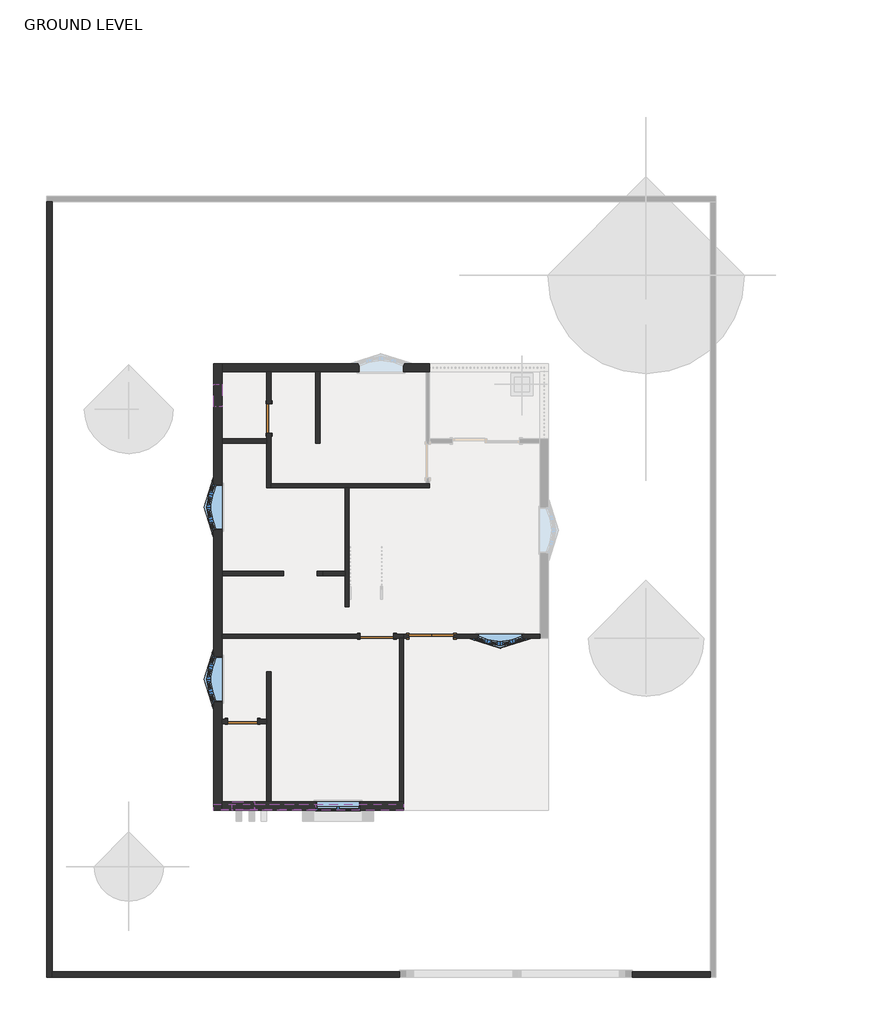
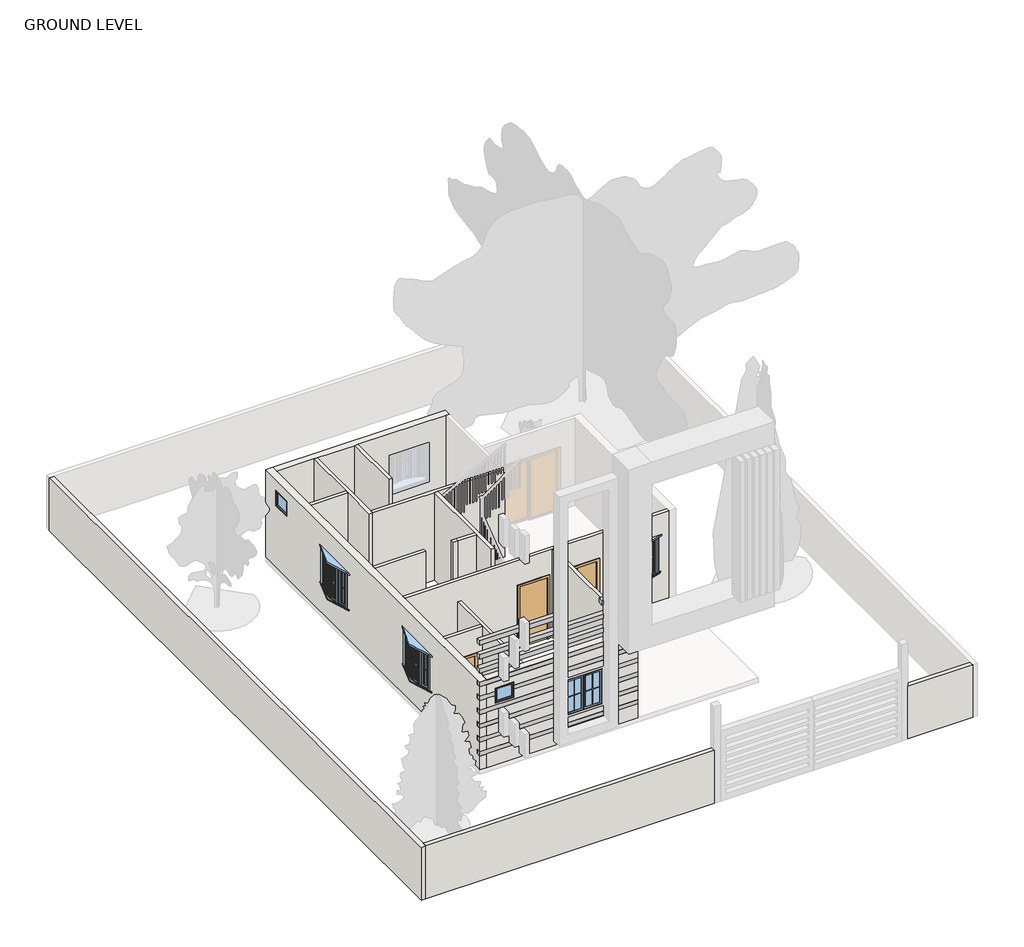
# One storey, part 1 of 3: 19 walls, 9 proxies, 6 windows, 4 doors.
"""IFC4 building model written with IfcOpenShell, lengths in millimetres."""

from ifc_helpers import new_model, si_unit, frame, origin, origin_with_axes, place, context, project, spatial, polyline, outline, extrude, faceted_brep, transform, mapped, element, save
from components import door_double_flush_panel_4_x7_eb8a45e1, door_d141acb4, door_38851409, single_flush_3_x7_305aa2a5, window_9e637e28, window_bow_casement_10_degree_angle_4_x4_fc1e5cf1, window_bow_casement_10_degree_angle_4_x4_a8433a54, window_casement_double_4_x4_af3140d2

model = new_model("IFC4")

# Units and contexts
model_context = context("Model", 3, world=origin())
ifc_project = project(units=[si_unit("LENGTHUNIT", "METRE", prefix="MILLI")], contexts=[model_context])

# Site, building, storey
site = spatial("IfcSite", under=ifc_project)
building = spatial("IfcBuilding", under=site)
storey = spatial("IfcBuildingStorey", under=building, Name="GROUND LEVEL", Elevation=0.0)

# Proxies
placement = place(None, origin())
element("IfcBuildingElementProxy", 1, Name="Reveal", ObjectType="Reveal", at=placement, inside=storey, context=model_context, shape_type="SweptSolid", body=[
    extrude(outline(polyline([(-1823.7720223, -5557.8064015), (-1823.7720223, -5405.4064015), (-645.6415084, -5405.4064015), (-645.6415084, -5557.8064015), (-1823.7720223, -5557.8064015)])), frame((0.0, 0.0, 4331.3684211), z_axis=(0.0, 0.0, 1.0), x_axis=(1.0, 0.0, 0.0)), (0.0, 0.0, 1.0), 152.4),
    extrude(outline(polyline([(-5827.2415084, -5557.8064015), (-5827.2415084, -5405.4064015), (-3042.9720223, -5405.4064015), (-3042.9720223, -5557.8064015), (-5827.2415084, -5557.8064015)])), frame((0.0, 0.0, 4331.3684211), z_axis=(0.0, 0.0, 1.0), x_axis=(1.0, 0.0, 0.0)), (0.0, 0.0, 1.0), 152.4),
])
element("IfcBuildingElementProxy", 2, Name="Reveal", ObjectType="Reveal", at=placement, inside=storey, context=model_context, shape_type="SweptSolid", body=[
    extrude(outline(polyline([(-5827.2415084, -5557.8064015), (-5827.2415084, -5405.4064015), (-645.6415084, -5405.4064015), (-645.6415084, -5557.8064015), (-5827.2415084, -5557.8064015)])), frame((0.0, 0.0, 3850.1052632), z_axis=(0.0, 0.0, 1.0), x_axis=(1.0, 0.0, 0.0)), (0.0, 0.0, 1.0), 152.4),
])
element("IfcBuildingElementProxy", 3, Name="Reveal", ObjectType="Reveal", at=placement, inside=storey, context=model_context, shape_type="SweptSolid", body=[
    extrude(outline(polyline([(-5827.2415084, -5557.8064015), (-5827.2415084, -5405.4064015), (-645.6415084, -5405.4064015), (-645.6415084, -5557.8064015), (-5827.2415084, -5557.8064015)])), frame((0.0, 0.0, 3368.8421053), z_axis=(0.0, 0.0, 1.0), x_axis=(1.0, 0.0, 0.0)), (0.0, 0.0, 1.0), 152.4),
])
element("IfcBuildingElementProxy", 4, Name="Reveal", ObjectType="Reveal", at=placement, inside=storey, context=model_context, shape_type="SweptSolid", body=[
    extrude(outline(polyline([(-5827.2415084, -5557.8064015), (-5827.2415084, -5405.4064015), (-645.6415084, -5405.4064015), (-645.6415084, -5557.8064015), (-5827.2415084, -5557.8064015)])), frame((0.0, 0.0, 2887.5789474), z_axis=(0.0, 0.0, 1.0), x_axis=(1.0, 0.0, 0.0)), (0.0, 0.0, 1.0), 152.4),
])
element("IfcBuildingElementProxy", 5, Name="Reveal", ObjectType="Reveal", at=placement, inside=storey, context=model_context, shape_type="SweptSolid", body=[
    extrude(outline(polyline([(-4712.8165084, -5557.8064015), (-4712.8165084, -5405.4064015), (-645.6415084, -5405.4064015), (-645.6415084, -5557.8064015), (-4712.8165084, -5557.8064015)])), frame((0.0, 0.0, 2406.3157895), z_axis=(0.0, 0.0, 1.0), x_axis=(1.0, 0.0, 0.0)), (0.0, 0.0, 1.0), 152.4),
    extrude(outline(polyline([(-5827.2415084, -5557.8064015), (-5827.2415084, -5405.4064015), (-5322.4165084, -5405.4064015), (-5322.4165084, -5557.8064015), (-5827.2415084, -5557.8064015)])), frame((0.0, 0.0, 2406.3157895), z_axis=(0.0, 0.0, 1.0), x_axis=(1.0, 0.0, 0.0)), (0.0, 0.0, 1.0), 152.4),
])
element("IfcBuildingElementProxy", 6, Name="Reveal", ObjectType="Reveal", at=placement, inside=storey, context=model_context, shape_type="SweptSolid", body=[
    extrude(outline(polyline([(-1823.7720223, -5557.8064015), (-1823.7720223, -5405.4064015), (-645.6415084, -5405.4064015), (-645.6415084, -5557.8064015), (-1823.7720223, -5557.8064015)])), frame((0.0, 0.0, 1925.0526316), z_axis=(0.0, 0.0, 1.0), x_axis=(1.0, 0.0, 0.0)), (0.0, 0.0, 1.0), 152.4),
    extrude(outline(polyline([(-5827.2415084, -5557.8064015), (-5827.2415084, -5405.4064015), (-3042.9720223, -5405.4064015), (-3042.9720223, -5557.8064015), (-5827.2415084, -5557.8064015)])), frame((0.0, 0.0, 1925.0526316), z_axis=(0.0, 0.0, 1.0), x_axis=(1.0, 0.0, 0.0)), (0.0, 0.0, 1.0), 152.4),
])
element("IfcBuildingElementProxy", 7, Name="Reveal", ObjectType="Reveal", at=placement, inside=storey, context=model_context, shape_type="SweptSolid", body=[
    extrude(outline(polyline([(-1823.7720223, -5557.8064015), (-1823.7720223, -5405.4064015), (-645.6415084, -5405.4064015), (-645.6415084, -5557.8064015), (-1823.7720223, -5557.8064015)])), frame((0.0, 0.0, 1443.7894737), z_axis=(0.0, 0.0, 1.0), x_axis=(1.0, 0.0, 0.0)), (0.0, 0.0, 1.0), 152.4),
    extrude(outline(polyline([(-5827.2415084, -5557.8064015), (-5827.2415084, -5405.4064015), (-3042.9720223, -5405.4064015), (-3042.9720223, -5557.8064015), (-5827.2415084, -5557.8064015)])), frame((0.0, 0.0, 1443.7894737), z_axis=(0.0, 0.0, 1.0), x_axis=(1.0, 0.0, 0.0)), (0.0, 0.0, 1.0), 152.4),
])
element("IfcBuildingElementProxy", 8, Name="Reveal", ObjectType="Reveal", at=placement, inside=storey, context=model_context, shape_type="SweptSolid", body=[
    extrude(outline(polyline([(-5827.2415084, -5557.8064015), (-5827.2415084, -5405.4064015), (-3042.9720223, -5405.4064015), (-3042.9720223, -5557.8064015), (-5827.2415084, -5557.8064015)])), frame((0.0, 0.0, 962.5263158), z_axis=(0.0, 0.0, 1.0), x_axis=(1.0, 0.0, 0.0)), (0.0, 0.0, 1.0), 152.4),
    extrude(outline(polyline([(-1823.7720223, -5557.8064015), (-1823.7720223, -5405.4064015), (-645.6415084, -5405.4064015), (-645.6415084, -5557.8064015), (-1823.7720223, -5557.8064015)])), frame((0.0, 0.0, 962.5263158), z_axis=(0.0, 0.0, 1.0), x_axis=(1.0, 0.0, 0.0)), (0.0, 0.0, 1.0), 152.4),
])
element("IfcBuildingElementProxy", 9, Name="Reveal", ObjectType="Reveal", at=placement, inside=storey, context=model_context, shape_type="SweptSolid", body=[
    extrude(outline(polyline([(-5827.2415084, -5557.8064015), (-5827.2415084, -5405.4064015), (-645.6415084, -5405.4064015), (-645.6415084, -5557.8064015), (-5827.2415084, -5557.8064015)])), frame((0.0, 0.0, 481.2631579), z_axis=(0.0, 0.0, 1.0), x_axis=(1.0, 0.0, 0.0)), (0.0, 0.0, 1.0), 152.4),
])

# Doors
door_double_flush_panel_4_x7_shape = door_double_flush_panel_4_x7_eb8a45e1(model_context)
element("IfcDoor", 10, ObjectType="Door-Double-Flush_Panel : 4'X7'", at=placement, inside=storey, context=model_context, shape_type="MappedRepresentation", body=[
    mapped(door_double_flush_panel_4_x7_shape, transform((116.3584916, -814.3564015, 0.0), x_axis=(1.0, 0.0, 0.0), y_axis=(0.0, 1.0, 0.0), z_axis=(0.0, 0.0, 1.0))),
])
door_shape = door_d141acb4(model_context)
element("IfcDoor", 11, ObjectType="Single-Flush : 2'8\"X7'", at=placement, inside=storey, context=model_context, shape_type="MappedRepresentation", body=[
    mapped(door_shape, transform((-5039.8415084, -3138.4564015, 0.0), x_axis=(-1.0, 0.0, 0.0), y_axis=(0.0, -1.0, 0.0), z_axis=(0.0, 0.0, 1.0))),
])
door_2_shape = door_38851409(model_context)
element("IfcDoor", 12, ObjectType="Single-Flush : 2'8\"X7'", at=placement, inside=storey, context=model_context, shape_type="MappedRepresentation", body=[
    mapped(door_2_shape, transform((-4322.2915084, 5135.5935985, 0.0), x_axis=(0.0, -1.0, 0.0), y_axis=(1.0, 0.0, 0.0), z_axis=(0.0, 0.0, 1.0))),
])
single_flush_3_x7_shape = single_flush_3_x7_305aa2a5(model_context)
element("IfcDoor", 13, ObjectType="Single-Flush : 3'X7'", at=placement, inside=storey, context=model_context, shape_type="MappedRepresentation", body=[
    mapped(single_flush_3_x7_shape, transform((-1369.5415084, -814.3564015, 0.0), x_axis=(1.0, 0.0, 0.0), y_axis=(0.0, 1.0, 0.0), z_axis=(0.0, 0.0, 1.0))),
])

# Walls
element("IfcWall", 14, ObjectType="4.5\"", at=placement, inside=storey, context=model_context, shape_type="Brep", body=[
    faceted_brep([(-912.3415084, -871.5064015, 2133.6), (-912.3415084, -871.5064015, 0.0), (-759.9415084, -871.5064015, 0.0), (-645.6415084, -871.5064015, 0.0), (-645.6415084, -871.5064015, 3048.0), (-759.9415084, -871.5064015, 3048.0), (-5598.6415084, -871.5064015, 3048.0), (-5598.6415084, -871.5064015, 0.0), (-1826.7415084, -871.5064015, 0.0), (-1826.7415084, -871.5064015, 2133.6), (-645.6415084, -757.2064015, 0.0), (-912.3415084, -757.2064015, 0.0), (-912.3415084, -757.2064015, 2133.6), (-1826.7415084, -757.2064015, 2133.6), (-1826.7415084, -757.2064015, 0.0), (-5598.6415084, -757.2064015, 0.0), (-5598.6415084, -757.2064015, 3048.0), (-645.6415084, -757.2064015, 3048.0)], [[[0, 1, 2, 3, 4, 5, 6, 7, 8, 9]], [[10, 11, 12, 13, 14, 15, 16, 17]], [[8, 7, 15, 14]], [[3, 2, 1, 11, 10]], [[6, 5, 4, 17, 16]], [[7, 6, 16, 15]], [[4, 3, 10, 17]], [[12, 11, 1, 0]], [[13, 12, 0, 9]], [[14, 13, 9, 8]]]),
])
element("IfcWall", 15, ObjectType="4.5\"", at=placement, inside=storey, context=model_context, shape_type="SweptSolid", body=[
    extrude(outline(polyline([(-759.9415084, -5329.2064015), (-759.9415084, -871.5064015), (-645.6415084, -871.5064015), (-645.6415084, -5329.2064015), (-759.9415084, -5329.2064015)])), origin_with_axes(), (0.0, 0.0, 1.0), 3048.0),
])
element("IfcWall", 16, ObjectType="4.5\"", at=placement, inside=storey, context=model_context, shape_type="Brep", body=[
    faceted_brep([(-645.6415084, -757.2064015, 3048.0), (3088.1584916, -757.2064015, 3048.0), (3088.1584916, -757.2064015, 0.0), (725.9584916, -757.2064015, 0.0), (725.9584916, -757.2064015, 2133.6), (-493.2415084, -757.2064015, 2133.6), (-493.2415084, -757.2064015, 0.0), (-645.6415084, -757.2064015, 0.0), (2603.2834745, -757.2064015, 2263.7323709), (1384.0834745, -757.2064015, 2263.7323709), (1384.0834745, -757.2064015, 993.7323709), (2603.2834745, -757.2064015, 993.7323709), (3088.1584916, -871.5064015, 3048.0), (-645.6415084, -871.5064015, 3048.0), (-645.6415084, -871.5064015, 0.0), (-493.2415084, -871.5064015, 0.0), (-493.2415084, -871.5064015, 2133.6), (725.9584916, -871.5064015, 2133.6), (725.9584916, -871.5064015, 0.0), (3088.1584916, -871.5064015, 0.0), (1360.1933675, -871.5064015, 2263.7323709), (2627.1735815, -871.5064015, 2263.7323709), (2627.1735815, -871.5064015, 993.7323709), (1360.1933675, -871.5064015, 993.7323709), (2603.2834745, -805.868872, 2263.7323709), (1384.0834745, -805.868872, 2263.7323709), (2603.2834745, -805.868872, 993.7323709), (1384.0834745, -805.868872, 993.7323709)], [[[0, 1, 2, 3, 4, 5, 6, 7], [8, 9, 10, 11]], [[12, 13, 14, 15, 16, 17, 18, 19], [20, 21, 22, 23]], [[2, 19, 18, 3]], [[14, 7, 6, 15]], [[1, 0, 13, 12]], [[2, 1, 12, 19]], [[0, 7, 14, 13]], [[17, 4, 3, 18]], [[4, 17, 16, 5]], [[5, 16, 15, 6]], [[24, 21, 20, 25, 9, 8]], [[26, 11, 10, 27, 23, 22]], [[24, 8, 11, 26]], [[9, 25, 27, 10]], [[25, 20, 23, 27]], [[21, 24, 26, 22]]]),
])
element("IfcWall", 17, ObjectType="4.5\"", at=placement, inside=storey, context=model_context, shape_type="SweptSolid", body=[
    extrude(outline(polyline([(-3045.9415084, 4462.4935985), (-3045.9415084, 6405.5935985), (-2931.6415084, 6405.5935985), (-2931.6415084, 4462.4935985), (-3045.9415084, 4462.4935985)])), origin_with_axes(), (0.0, 0.0, 1.0), 3048.0),
])
element("IfcWall", 18, ObjectType="4.5\"", at=placement, inside=storey, context=model_context, shape_type="Brep", body=[
    faceted_brep([(-4379.4415084, 4729.1935985, 2133.6), (-4379.4415084, 4729.1935985, 0.0), (-4379.4415084, 4576.7935985, 0.0), (-4379.4415084, 4462.4935985, 0.0), (-4379.4415084, 3243.2935985, 0.0), (-4379.4415084, 3243.2935985, 3048.0), (-4379.4415084, 4462.4935985, 3048.0), (-4379.4415084, 4576.7935985, 3048.0), (-4379.4415084, 6405.5935985, 3048.0), (-4379.4415084, 6405.5935985, 0.0), (-4379.4415084, 5541.9935985, 0.0), (-4379.4415084, 5541.9935985, 2133.6), (-4265.1415084, 3243.2935985, 0.0), (-4265.1415084, 3357.5935985, 0.0), (-4265.1415084, 4729.1935985, 0.0), (-4265.1415084, 4729.1935985, 2133.6), (-4265.1415084, 5541.9935985, 2133.6), (-4265.1415084, 5541.9935985, 0.0), (-4265.1415084, 6405.5935985, 0.0), (-4265.1415084, 6405.5935985, 3048.0), (-4265.1415084, 3357.5935985, 3048.0), (-4265.1415084, 3243.2935985, 3048.0)], [[[0, 1, 2, 3, 4, 5, 6, 7, 8, 9, 10, 11]], [[12, 13, 14, 15, 16, 17, 18, 19, 20, 21]], [[10, 9, 18, 17]], [[4, 3, 2, 1, 14, 13, 12]], [[8, 7, 6, 5, 21, 20, 19]], [[9, 8, 19, 18]], [[5, 4, 12, 21]], [[15, 14, 1, 0]], [[16, 15, 0, 11]], [[17, 16, 11, 10]]]),
])
element("IfcWall", 19, ObjectType="4.5\"", at=placement, inside=storey, context=model_context, shape_type="SweptSolid", body=[
    extrude(outline(polyline([(-5598.6415084, 4576.7935985), (-4379.4415084, 4576.7935985), (-4379.4415084, 4462.4935985), (-5598.6415084, 4462.4935985), (-5598.6415084, 4576.7935985)])), origin_with_axes(), (0.0, 0.0, 1.0), 3048.0),
])
element("IfcWall", 20, ObjectType="4.5\"", at=placement, inside=storey, context=model_context, shape_type="Brep", body=[
    faceted_brep([(-4265.1415084, 3243.2935985, 0.0), (-2245.8415084, 3243.2935985, 0.0), (-2131.5415084, 3243.2935985, 0.0), (65.5584916, 3243.2935985, 0.0), (65.5584916, 3243.2935985, 3048.0), (-2131.5415084, 3243.2935985, 3048.0), (-2245.8415084, 3243.2935985, 3048.0), (-4265.1415084, 3243.2935985, 3048.0), (-4265.1415084, 3357.5935985, 0.0), (-4265.1415084, 3357.5935985, 3048.0), (-36.0415084, 3357.5935985, 3048.0), (65.5584916, 3357.5935985, 3048.0), (65.5584916, 3357.5935985, 0.0), (-36.0415084, 3357.5935985, 0.0)], [[[0, 1, 2, 3, 4, 5, 6, 7]], [[8, 9, 10, 11, 12, 13]], [[3, 2, 1, 0, 8, 13, 12]], [[7, 6, 5, 4, 11, 10, 9]], [[0, 7, 9, 8]], [[4, 3, 12, 11]]]),
])
element("IfcWall", 21, ObjectType="4.5\"", at=placement, inside=storey, context=model_context, shape_type="SweptSolid", body=[
    extrude(outline(polyline([(-3922.2415084, 842.9935985), (-5598.6415084, 842.9935985), (-5598.6415084, 957.2935985), (-3922.2415084, 957.2935985), (-3922.2415084, 842.9935985)])), origin_with_axes(), (0.0, 0.0, 1.0), 3048.0),
])
element("IfcWall", 22, ObjectType="4.5\"", at=placement, inside=storey, context=model_context, shape_type="SweptSolid", body=[
    extrude(outline(polyline([(-3007.8415084, 957.2935985), (-2855.4415084, 957.2935985), (-2855.4415084, 842.9935985), (-3007.8415084, 842.9935985), (-3007.8415084, 957.2935985)])), origin_with_axes(), (0.0, 0.0, 1.0), 3048.0),
])
element("IfcWall", 23, ObjectType="4.5\"", at=placement, inside=storey, context=model_context, shape_type="Brep", body=[
    faceted_brep([(-2245.8415084, 3243.2935985, 0.0), (-2245.8415084, 957.2935985, 0.0), (-2245.8415084, 842.9935985, 0.0), (-2245.8415084, -9.4533727, 0.0), (-2245.8415084, -9.4533727, 3048.0), (-2245.8415084, 842.9935985, 3048.0), (-2245.8415084, 957.2935985, 3048.0), (-2245.8415084, 3243.2935985, 3048.0), (-2131.5415084, 3243.2935985, 0.0), (-2131.5415084, 3243.2935985, 3048.0), (-2131.5415084, -9.4533727, 3048.0), (-2131.5415084, -9.4533727, 0.0)], [[[0, 1, 2, 3, 4, 5, 6, 7]], [[8, 9, 10, 11]], [[3, 2, 1, 0, 8, 11]], [[4, 3, 11, 10]], [[7, 6, 5, 4, 10, 9]], [[0, 7, 9, 8]]]),
])
element("IfcWall", 24, ObjectType="4.5\"", at=placement, inside=storey, context=model_context, shape_type="SweptSolid", body=[
    extrude(outline(polyline([(-2245.8415084, 842.9935985), (-2855.4415084, 842.9935985), (-2855.4415084, 957.2935985), (-2245.8415084, 957.2935985), (-2245.8415084, 842.9935985)])), origin_with_axes(), (0.0, 0.0, 1.0), 3048.0),
])
element("IfcWall", 25, ObjectType="4.5\"", at=placement, inside=storey, context=model_context, shape_type="Brep", body=[
    faceted_brep([(-4265.1415084, -5329.2064015, 0.0), (-4265.1415084, -1785.9064015, 0.0), (-4265.1415084, -1785.9064015, 3048.0), (-4265.1415084, -5329.2064015, 3048.0), (-4379.4415084, -5329.2064015, 0.0), (-4379.4415084, -5329.2064015, 3048.0), (-4379.4415084, -3195.6064015, 3048.0), (-4379.4415084, -3081.3064015, 3048.0), (-4379.4415084, -1785.9064015, 3048.0), (-4379.4415084, -1785.9064015, 0.0), (-4379.4415084, -3081.3064015, 0.0), (-4379.4415084, -3195.6064015, 0.0)], [[[0, 1, 2, 3]], [[4, 5, 6, 7, 8, 9, 10, 11]], [[1, 0, 4, 11, 10, 9]], [[2, 1, 9, 8]], [[3, 2, 8, 7, 6, 5]], [[0, 3, 5, 4]]]),
])
element("IfcWall", 26, ObjectType="4.5\"", at=placement, inside=storey, context=model_context, shape_type="SweptSolid", body=[
    extrude(outline(polyline([(0.0, -5598.6415084), (0.0, -5446.2415084), (2133.6, -5446.2415084), (2133.6, -4633.4415084), (0.0, -4633.4415084), (0.0, -4379.4415084), (3048.0, -4379.4415084), (3048.0, -5598.6415084), (0.0, -5598.6415084)])), frame((0.0, -3195.6064015, 0.0), z_axis=(0.0, 1.0, 0.0), x_axis=(0.0, 0.0, 1.0)), (0.0, 0.0, 1.0), 114.3),
])
element("IfcWall", 27, ObjectType="6\"", at=placement, inside=storey, context=model_context, shape_type="Brep", body=[
    faceted_brep([(-10399.2415084, 11053.7935985, -152.4), (-10399.2415084, -10129.8064015, -152.4), (-10399.2415084, -10129.8064015, 1676.4), (-10399.2415084, 11053.7935985, 1676.4), (-10246.8415084, 11053.7935985, -152.4), (-10246.8415084, 11053.7935985, 1676.4), (-10246.8415084, -9977.4064015, 1676.4), (-10246.8415084, -10129.8064015, 1676.4), (-10246.8415084, -10129.8064015, -152.4), (-10246.8415084, -9977.4064015, -152.4)], [[[0, 1, 2, 3]], [[4, 5, 6, 7, 8, 9]], [[1, 0, 4, 9, 8]], [[3, 2, 7, 6, 5]], [[0, 3, 5, 4]], [[2, 1, 8, 7]]]),
])
element("IfcWall", 28, ObjectType="6\"", at=placement, inside=storey, context=model_context, shape_type="SweptSolid", body=[
    extrude(outline(polyline([(-759.9415084, -10129.8064015), (-10246.8415084, -10129.8064015), (-10246.8415084, -9977.4064015), (-759.9415084, -9977.4064015), (-759.9415084, -10129.8064015)])), frame((0.0, 0.0, -152.4), z_axis=(0.0, 0.0, 1.0), x_axis=(1.0, 0.0, 0.0)), (0.0, 0.0, 1.0), 1828.8),
])
element("IfcWall", 29, ObjectType="6\"", at=placement, inside=storey, context=model_context, shape_type="SweptSolid", body=[
    extrude(outline(polyline([(5602.7584916, -9977.4064015), (7736.3584916, -9977.4064015), (7736.3584916, -10129.8064015), (5602.7584916, -10129.8064015), (5602.7584916, -9977.4064015)])), frame((0.0, 0.0, -152.4), z_axis=(0.0, 0.0, 1.0), x_axis=(1.0, 0.0, 0.0)), (0.0, 0.0, 1.0), 1828.8),
])
element("IfcWall", 30, ObjectType="9\"", at=placement, inside=storey, context=model_context, shape_type="Brep", body=[
    faceted_brep([(-5827.2415084, 6634.1935985, 0.0), (-5827.2415084, -5557.8064015, 0.0), (-5827.2415084, -5557.8064015, 481.2631579), (-5827.2415084, -5405.4064015, 481.2631579), (-5827.2415084, -5405.4064015, 633.6631579), (-5827.2415084, -5557.8064015, 633.6631579), (-5827.2415084, -5557.8064015, 962.5263158), (-5827.2415084, -5405.4064015, 962.5263158), (-5827.2415084, -5405.4064015, 1114.9263158), (-5827.2415084, -5557.8064015, 1114.9263158), (-5827.2415084, -5557.8064015, 1443.7894737), (-5827.2415084, -5405.4064015, 1443.7894737), (-5827.2415084, -5405.4064015, 1596.1894737), (-5827.2415084, -5557.8064015, 1596.1894737), (-5827.2415084, -5557.8064015, 1925.0526316), (-5827.2415084, -5405.4064015, 1925.0526316), (-5827.2415084, -5405.4064015, 2077.4526316), (-5827.2415084, -5557.8064015, 2077.4526316), (-5827.2415084, -5557.8064015, 2406.3157895), (-5827.2415084, -5405.4064015, 2406.3157895), (-5827.2415084, -5405.4064015, 2558.7157895), (-5827.2415084, -5557.8064015, 2558.7157895), (-5827.2415084, -5557.8064015, 2887.5789474), (-5827.2415084, -5405.4064015, 2887.5789474), (-5827.2415084, -5405.4064015, 3039.9789474), (-5827.2415084, -5557.8064015, 3039.9789474), (-5827.2415084, -5557.8064015, 3048.0), (-5827.2415084, 6634.1935985, 3048.0), (-5827.2415084, 6062.6935985, 2133.6), (-5827.2415084, 6062.6935985, 2667.0), (-5827.2415084, 5453.0935985, 2667.0), (-5827.2415084, 5453.0935985, 2133.6), (-5827.2415084, -1354.6176736, 2263.7323709), (-5827.2415084, -2621.5978876, 2263.7323709), (-5827.2415084, -2621.5978876, 993.7323709), (-5827.2415084, -1354.6176736, 993.7323709), (-5827.2415084, 3342.0645075, 2263.7323709), (-5827.2415084, 2075.0842935, 2263.7323709), (-5827.2415084, 2075.0842935, 993.7323709), (-5827.2415084, 3342.0645075, 993.7323709), (-5598.6415084, -5557.8064015, 0.0), (-5598.6415084, -5329.2064015, 0.0), (-5598.6415084, -3195.6064015, 0.0), (-5598.6415084, -3081.3064015, 0.0), (-5598.6415084, -871.5064015, 0.0), (-5598.6415084, -757.2064015, 0.0), (-5598.6415084, 842.9935985, 0.0), (-5598.6415084, 957.2935985, 0.0), (-5598.6415084, 4462.4935985, 0.0), (-5598.6415084, 4576.7935985, 0.0), (-5598.6415084, 6405.5935985, 0.0), (-5598.6415084, 6634.1935985, 0.0), (-5598.6415084, 6634.1935985, 3048.0), (-5598.6415084, 6405.5935985, 3048.0), (-5598.6415084, 4576.7935985, 3048.0), (-5598.6415084, 4462.4935985, 3048.0), (-5598.6415084, 957.2935985, 3048.0), (-5598.6415084, 842.9935985, 3048.0), (-5598.6415084, -757.2064015, 3048.0), (-5598.6415084, -871.5064015, 3048.0), (-5598.6415084, -3081.3064015, 3048.0), (-5598.6415084, -3195.6064015, 3048.0), (-5598.6415084, -5329.2064015, 3048.0), (-5598.6415084, -5557.8064015, 3048.0), (-5598.6415084, -5557.8064015, 3039.9789474), (-5598.6415084, -5405.4064015, 3039.9789474), (-5598.6415084, -5405.4064015, 2887.5789474), (-5598.6415084, -5557.8064015, 2887.5789474), (-5598.6415084, -5557.8064015, 2558.7157895), (-5598.6415084, -5405.4064015, 2558.7157895), (-5598.6415084, -5405.4064015, 2406.3157895), (-5598.6415084, -5557.8064015, 2406.3157895), (-5598.6415084, -5557.8064015, 2077.4526316), (-5598.6415084, -5405.4064015, 2077.4526316), (-5598.6415084, -5405.4064015, 1925.0526316), (-5598.6415084, -5557.8064015, 1925.0526316), (-5598.6415084, -5557.8064015, 1596.1894737), (-5598.6415084, -5405.4064015, 1596.1894737), (-5598.6415084, -5405.4064015, 1443.7894737), (-5598.6415084, -5557.8064015, 1443.7894737), (-5598.6415084, -5557.8064015, 1114.9263158), (-5598.6415084, -5405.4064015, 1114.9263158), (-5598.6415084, -5405.4064015, 962.5263158), (-5598.6415084, -5557.8064015, 962.5263158), (-5598.6415084, -5557.8064015, 633.6631579), (-5598.6415084, -5405.4064015, 633.6631579), (-5598.6415084, -5405.4064015, 481.2631579), (-5598.6415084, -5557.8064015, 481.2631579), (-5598.6415084, 6062.6935985, 2667.0), (-5598.6415084, 6062.6935985, 2133.6), (-5598.6415084, 5453.0935985, 2133.6), (-5598.6415084, 5453.0935985, 2667.0), (-5598.6415084, -2597.7077806, 2263.7323709), (-5598.6415084, -1378.5077806, 2263.7323709), (-5598.6415084, -1378.5077806, 993.7323709), (-5598.6415084, -2597.7077806, 993.7323709), (-5598.6415084, 2098.9744005, 2263.7323709), (-5598.6415084, 3318.1744005, 2263.7323709), (-5598.6415084, 3318.1744005, 993.7323709), (-5598.6415084, 2098.9744005, 993.7323709), (-5761.6039788, -2597.7077806, 2263.7323709), (-5761.6039788, -1378.5077806, 2263.7323709), (-5761.6039788, -2597.7077806, 993.7323709), (-5761.6039788, -1378.5077806, 993.7323709), (-5761.6039788, 2098.9744005, 2263.7323709), (-5761.6039788, 3318.1744005, 2263.7323709), (-5761.6039788, 2098.9744005, 993.7323709), (-5761.6039788, 3318.1744005, 993.7323709)], [[[0, 1, 2, 3, 4, 5, 6, 7, 8, 9, 10, 11, 12, 13, 14, 15, 16, 17, 18, 19, 20, 21, 22, 23, 24, 25, 26, 27], [28, 29, 30, 31], [32, 33, 34, 35], [36, 37, 38, 39]], [[40, 41, 42, 43, 44, 45, 46, 47, 48, 49, 50, 51, 52, 53, 54, 55, 56, 57, 58, 59, 60, 61, 62, 63, 64, 65, 66, 67, 68, 69, 70, 71, 72, 73, 74, 75, 76, 77, 78, 79, 80, 81, 82, 83, 84, 85, 86, 87], [88, 89, 90, 91], [92, 93, 94, 95], [96, 97, 98, 99]], [[1, 0, 51, 50, 49, 48, 47, 46, 45, 44, 43, 42, 41, 40]], [[27, 26, 63, 62, 61, 60, 59, 58, 57, 56, 55, 54, 53, 52]], [[1, 40, 87, 2]], [[63, 26, 25, 64]], [[5, 84, 83, 6]], [[9, 80, 79, 10]], [[13, 76, 75, 14]], [[17, 72, 71, 18]], [[21, 68, 67, 22]], [[0, 27, 52, 51]], [[89, 88, 29, 28]], [[90, 89, 28, 31]], [[91, 90, 31, 30]], [[88, 91, 30, 29]], [[100, 33, 32, 101, 93, 92]], [[102, 95, 94, 103, 35, 34]], [[100, 92, 95, 102]], [[93, 101, 103, 94]], [[101, 32, 35, 103]], [[33, 100, 102, 34]], [[104, 37, 36, 105, 97, 96]], [[106, 99, 98, 107, 39, 38]], [[104, 96, 99, 106]], [[97, 105, 107, 98]], [[105, 36, 39, 107]], [[37, 104, 106, 38]], [[4, 85, 84, 5]], [[85, 4, 3, 86]], [[86, 3, 2, 87]], [[8, 81, 80, 9]], [[81, 8, 7, 82]], [[82, 7, 6, 83]], [[12, 77, 76, 13]], [[77, 12, 11, 78]], [[78, 11, 10, 79]], [[16, 73, 72, 17]], [[73, 16, 15, 74]], [[74, 15, 14, 75]], [[20, 69, 68, 21]], [[69, 20, 19, 70]], [[70, 19, 18, 71]], [[24, 65, 64, 25]], [[65, 24, 23, 66]], [[66, 23, 22, 67]]]),
])
element("IfcWall", 31, ObjectType="9\"", at=placement, inside=storey, context=model_context, shape_type="Brep", body=[
    faceted_brep([(-5598.6415084, -5557.8064015, 0.0), (-645.6415084, -5557.8064015, 0.0), (-645.6415084, -5557.8064015, 481.2631579), (-5598.6415084, -5557.8064015, 481.2631579), (-645.6415084, -5557.8064015, 3048.0), (-5598.6415084, -5557.8064015, 3048.0), (-5598.6415084, -5557.8064015, 3039.9789474), (-645.6415084, -5557.8064015, 3039.9789474), (-4712.8165084, -5557.8064015, 2133.6), (-5322.4165084, -5557.8064015, 2133.6), (-5322.4165084, -5557.8064015, 2406.3157895), (-5598.6415084, -5557.8064015, 2406.3157895), (-5598.6415084, -5557.8064015, 2077.4526316), (-3042.9720223, -5557.8064015, 2077.4526316), (-3042.9720223, -5557.8064015, 2133.6), (-1823.7720223, -5557.8064015, 2133.6), (-1823.7720223, -5557.8064015, 2077.4526316), (-645.6415084, -5557.8064015, 2077.4526316), (-645.6415084, -5557.8064015, 2406.3157895), (-4712.8165084, -5557.8064015, 2406.3157895), (-5322.4165084, -5557.8064015, 2667.0), (-4712.8165084, -5557.8064015, 2667.0), (-4712.8165084, -5557.8064015, 2558.7157895), (-645.6415084, -5557.8064015, 2558.7157895), (-645.6415084, -5557.8064015, 2887.5789474), (-5598.6415084, -5557.8064015, 2887.5789474), (-5598.6415084, -5557.8064015, 2558.7157895), (-5322.4165084, -5557.8064015, 2558.7157895), (-1823.7720223, -5557.8064015, 914.4), (-3042.9720223, -5557.8064015, 914.4), (-3042.9720223, -5557.8064015, 962.5263158), (-5598.6415084, -5557.8064015, 962.5263158), (-5598.6415084, -5557.8064015, 633.6631579), (-645.6415084, -5557.8064015, 633.6631579), (-645.6415084, -5557.8064015, 962.5263158), (-1823.7720223, -5557.8064015, 962.5263158), (-5598.6415084, -5557.8064015, 1114.9263158), (-3042.9720223, -5557.8064015, 1114.9263158), (-3042.9720223, -5557.8064015, 1443.7894737), (-5598.6415084, -5557.8064015, 1443.7894737), (-645.6415084, -5557.8064015, 1114.9263158), (-645.6415084, -5557.8064015, 1443.7894737), (-1823.7720223, -5557.8064015, 1443.7894737), (-1823.7720223, -5557.8064015, 1114.9263158), (-1823.7720223, -5557.8064015, 1596.1894737), (-645.6415084, -5557.8064015, 1596.1894737), (-645.6415084, -5557.8064015, 1925.0526316), (-1823.7720223, -5557.8064015, 1925.0526316), (-5598.6415084, -5557.8064015, 1596.1894737), (-3042.9720223, -5557.8064015, 1596.1894737), (-3042.9720223, -5557.8064015, 1925.0526316), (-5598.6415084, -5557.8064015, 1925.0526316), (-645.6415084, -5329.2064015, 0.0), (-759.9415084, -5329.2064015, 0.0), (-4265.1415084, -5329.2064015, 0.0), (-4379.4415084, -5329.2064015, 0.0), (-5598.6415084, -5329.2064015, 0.0), (-5598.6415084, -5329.2064015, 3048.0), (-4379.4415084, -5329.2064015, 3048.0), (-4265.1415084, -5329.2064015, 3048.0), (-759.9415084, -5329.2064015, 3048.0), (-645.6415084, -5329.2064015, 3048.0), (-5322.4165084, -5329.2064015, 2667.0), (-5322.4165084, -5329.2064015, 2133.6), (-4712.8165084, -5329.2064015, 2133.6), (-4712.8165084, -5329.2064015, 2667.0), (-3042.9720223, -5329.2064015, 2133.6), (-3042.9720223, -5329.2064015, 914.4), (-1823.7720223, -5329.2064015, 914.4), (-1823.7720223, -5329.2064015, 2133.6), (-5598.6415084, -5405.4064015, 481.2631579), (-5598.6415084, -5405.4064015, 633.6631579), (-5598.6415084, -5405.4064015, 962.5263158), (-5598.6415084, -5405.4064015, 1114.9263158), (-5598.6415084, -5405.4064015, 1443.7894737), (-5598.6415084, -5405.4064015, 1596.1894737), (-5598.6415084, -5405.4064015, 1925.0526316), (-5598.6415084, -5405.4064015, 2077.4526316), (-5598.6415084, -5405.4064015, 2406.3157895), (-5598.6415084, -5405.4064015, 2558.7157895), (-5598.6415084, -5405.4064015, 2887.5789474), (-5598.6415084, -5405.4064015, 3039.9789474), (-645.6415084, -5405.4064015, 3039.9789474), (-645.6415084, -5405.4064015, 2887.5789474), (-645.6415084, -5405.4064015, 2558.7157895), (-645.6415084, -5405.4064015, 2406.3157895), (-645.6415084, -5405.4064015, 2077.4526316), (-645.6415084, -5405.4064015, 1925.0526316), (-645.6415084, -5405.4064015, 1596.1894737), (-645.6415084, -5405.4064015, 1443.7894737), (-645.6415084, -5405.4064015, 1114.9263158), (-645.6415084, -5405.4064015, 962.5263158), (-645.6415084, -5405.4064015, 633.6631579), (-645.6415084, -5405.4064015, 481.2631579), (-5322.4165084, -5405.4064015, 2558.7157895), (-5322.4165084, -5405.4064015, 2406.3157895), (-4712.8165084, -5405.4064015, 2406.3157895), (-4712.8165084, -5405.4064015, 2558.7157895), (-3042.9720223, -5405.4064015, 2077.4526316), (-3042.9720223, -5405.4064015, 1925.0526316), (-3042.9720223, -5405.4064015, 1596.1894737), (-3042.9720223, -5405.4064015, 1443.7894737), (-3042.9720223, -5405.4064015, 1114.9263158), (-3042.9720223, -5405.4064015, 962.5263158), (-1823.7720223, -5405.4064015, 962.5263158), (-1823.7720223, -5405.4064015, 1114.9263158), (-1823.7720223, -5405.4064015, 1443.7894737), (-1823.7720223, -5405.4064015, 1596.1894737), (-1823.7720223, -5405.4064015, 1925.0526316), (-1823.7720223, -5405.4064015, 2077.4526316)], [[[0, 1, 2, 3]], [[4, 5, 6, 7]], [[8, 9, 10, 11, 12, 13, 14, 15, 16, 17, 18, 19]], [[20, 21, 22, 23, 24, 25, 26, 27]], [[28, 29, 30, 31, 32, 33, 34, 35]], [[36, 37, 38, 39]], [[40, 41, 42, 43]], [[44, 45, 46, 47]], [[48, 49, 50, 51]], [[52, 53, 54, 55, 56, 57, 58, 59, 60, 61], [62, 63, 64, 65], [66, 67, 68, 69]], [[1, 0, 56, 55, 54, 53, 52]], [[5, 4, 61, 60, 59, 58, 57]], [[5, 57, 56, 0, 3, 70, 71, 32, 31, 72, 73, 36, 39, 74, 75, 48, 51, 76, 77, 12, 11, 78, 79, 26, 25, 80, 81, 6]], [[1, 52, 61, 4, 7, 82, 83, 24, 23, 84, 85, 18, 17, 86, 87, 46, 45, 88, 89, 41, 40, 90, 91, 34, 33, 92, 93, 2]], [[63, 62, 20, 27, 94, 95, 10, 9]], [[64, 63, 9, 8]], [[65, 64, 8, 19, 96, 97, 22, 21]], [[62, 65, 21, 20]], [[67, 66, 14, 13, 98, 99, 50, 49, 100, 101, 38, 37, 102, 103, 30, 29]], [[29, 28, 68, 67]], [[69, 68, 28, 35, 104, 105, 43, 42, 106, 107, 44, 47, 108, 109, 16, 15]], [[71, 92, 33, 32]], [[92, 71, 70, 93]], [[93, 70, 3, 2]], [[73, 102, 37, 36]], [[102, 73, 72, 103]], [[103, 72, 31, 30]], [[107, 88, 45, 44]], [[88, 107, 106, 89]], [[89, 106, 42, 41]], [[75, 100, 49, 48]], [[100, 75, 74, 101]], [[101, 74, 39, 38]], [[109, 86, 17, 16]], [[86, 109, 108, 87]], [[87, 108, 47, 46]], [[77, 98, 13, 12]], [[98, 77, 76, 99]], [[99, 76, 51, 50]], [[97, 84, 23, 22]], [[84, 97, 96, 85]], [[85, 96, 19, 18]], [[79, 94, 27, 26]], [[94, 79, 78, 95]], [[95, 78, 11, 10]], [[81, 82, 7, 6]], [[82, 81, 80, 83]], [[83, 80, 25, 24]], [[14, 66, 69, 15]], [[105, 90, 40, 43]], [[90, 105, 104, 91]], [[91, 104, 35, 34]]]),
])
element("IfcWall", 32, ObjectType="9\"", at=placement, inside=storey, context=model_context, shape_type="Brep", body=[
    faceted_brep([(65.5584916, 6634.1935985, 3048.0), (65.5584916, 6634.1935985, 609.6), (65.5584916, 6634.1935985, 0.0), (-5598.6415084, 6634.1935985, 0.0), (-5598.6415084, 6634.1935985, 3048.0), (-621.7514014, 6634.1935985, 2263.7323709), (-1888.7316154, 6634.1935985, 2263.7323709), (-1888.7316154, 6634.1935985, 993.7323709), (-621.7514014, 6634.1935985, 993.7323709), (65.5584916, 6405.5935985, 0.0), (65.5584916, 6405.5935985, 609.6), (65.5584916, 6405.5935985, 3048.0), (-36.0415084, 6405.5935985, 3048.0), (-2931.6415084, 6405.5935985, 3048.0), (-3045.9415084, 6405.5935985, 3048.0), (-4265.1415084, 6405.5935985, 3048.0), (-4379.4415084, 6405.5935985, 3048.0), (-5598.6415084, 6405.5935985, 3048.0), (-5598.6415084, 6405.5935985, 0.0), (-4379.4415084, 6405.5935985, 0.0), (-4265.1415084, 6405.5935985, 0.0), (-3045.9415084, 6405.5935985, 0.0), (-2931.6415084, 6405.5935985, 0.0), (-36.0415084, 6405.5935985, 0.0), (-1864.8415084, 6405.5935985, 2263.7323709), (-645.6415084, 6405.5935985, 2263.7323709), (-645.6415084, 6405.5935985, 993.7323709), (-1864.8415084, 6405.5935985, 993.7323709), (-1864.8415084, 6568.5560689, 2263.7323709), (-645.6415084, 6568.5560689, 2263.7323709), (-1864.8415084, 6568.5560689, 993.7323709), (-645.6415084, 6568.5560689, 993.7323709)], [[[0, 1, 2, 3, 4], [5, 6, 7, 8]], [[9, 10, 11, 12, 13, 14, 15, 16, 17, 18, 19, 20, 21, 22, 23], [24, 25, 26, 27]], [[3, 2, 9, 23, 22, 21, 20, 19, 18]], [[0, 4, 17, 16, 15, 14, 13, 12, 11]], [[4, 3, 18, 17]], [[28, 6, 5, 29, 25, 24]], [[30, 27, 26, 31, 8, 7]], [[28, 24, 27, 30]], [[25, 29, 31, 26]], [[29, 5, 8, 31]], [[6, 28, 30, 7]], [[0, 11, 10, 9, 2, 1]]]),
])

# Windows
window_shape = window_9e637e28(model_context)
element("IfcWindow", 33, ObjectType="Fixed : 2'X1'9\"", at=placement, inside=storey, context=model_context, shape_type="MappedRepresentation", body=[
    mapped(window_shape, transform((-5055.7165084, -5443.5064015, 0.0), x_axis=(-1.0, 0.0, 0.0), y_axis=(0.0, -1.0, 0.0), z_axis=(0.0, 0.0, 1.0))),
])
element("IfcWindow", 34, ObjectType="Fixed : 2'X1'9\"", at=placement, inside=storey, context=model_context, shape_type="MappedRepresentation", body=[
    mapped(window_shape, transform((-5712.9415084, 5795.9935985, 0.0), x_axis=(0.0, 1.0, 0.0), y_axis=(-1.0, 0.0, 0.0), z_axis=(0.0, 0.0, 1.0))),
])
window_bow_casement_10_degree_angle_4_x4_shape = window_bow_casement_10_degree_angle_4_x4_fc1e5cf1(model_context)
element("IfcWindow", 35, ObjectType="Window-Bow-Casement-10_Degree_Angle : 4'X4'", at=placement, inside=storey, context=model_context, shape_type="MappedRepresentation", body=[
    mapped(window_bow_casement_10_degree_angle_4_x4_shape, transform((-5712.9415084, -1988.1077806, 384.1323709), x_axis=(0.0, 1.0, 0.0), y_axis=(-1.0, 0.0, 0.0), z_axis=(0.0, 0.0, 1.0))),
])
element("IfcWindow", 36, ObjectType="Window-Bow-Casement-10_Degree_Angle : 4'X4'", at=placement, inside=storey, context=model_context, shape_type="MappedRepresentation", body=[
    mapped(window_bow_casement_10_degree_angle_4_x4_shape, transform((-5712.9415084, 2708.5744005, 384.1323709), x_axis=(0.0, 1.0, 0.0), y_axis=(-1.0, 0.0, 0.0), z_axis=(0.0, 0.0, 1.0))),
])
window_bow_casement_10_degree_angle_4_x4_2_shape = window_bow_casement_10_degree_angle_4_x4_a8433a54(model_context)
element("IfcWindow", 37, ObjectType="Window-Bow-Casement-10_Degree_Angle : 4'X4'", at=placement, inside=storey, context=model_context, shape_type="MappedRepresentation", body=[
    mapped(window_bow_casement_10_degree_angle_4_x4_2_shape, transform((1993.6834745, -814.3564015, 384.1323709), x_axis=(-1.0, 0.0, 0.0), y_axis=(0.0, -1.0, 0.0), z_axis=(0.0, 0.0, 1.0))),
])
window_casement_double_4_x4_shape = window_casement_double_4_x4_af3140d2(model_context)
element("IfcWindow", 38, ObjectType="Window-Casement-Double : 4'X4'", at=placement, inside=storey, context=model_context, shape_type="MappedRepresentation", body=[
    mapped(window_casement_double_4_x4_shape, transform((-2433.3720223, -5443.5064015, 0.0), x_axis=(-1.0, 0.0, 0.0), y_axis=(0.0, -1.0, 0.0), z_axis=(0.0, 0.0, 1.0))),
])

save(model, "model.ifc")

# Revit data of these elements
# Type "Door-Double-Flush_Panel : 4'X7'"
#   Type Mark = "11"
#   Construction Type Id = "DOOR"
#   Assembly Code = "C1020"
#   Analytic Construction = "Wooden"
#   Thickness = 0' - 2"
#   Thermal Resistance (R) = 2.5876 (h·ft²·°F)/BTU
#   Swing Angle [instance default] = 90.00°
#   Panel Width = 2' - 0"
#   Heat Transfer Coefficient (U) = 0.3865 BTU/(h·ft²·°F)
#   Height = 7' - 0"
#   Trim Projection Ext = 0' - 1"
#   Trim Projection Int = 0' - 1"
#   Trim Width = 0' - 3"
#   Width = 4' - 0"
#   Define Thermal Properties by = 1
#   Panel Material = Wood - Birch - Solid Stained Light Low Gloss
#   Trim Material = Paint - Sienna
#   Visual Light Transmittance = 0
#   Solar Heat Gain Coefficient = 0
#   Function = (empty or 0)
#   Wall Closure = (empty or 0)
# Type "Single-Flush : 2'8\"X7'"
#   Type Mark = "9"
#   Construction Type Id = "MDOOR"
#   Assembly Code = "C1020"
#   Analytic Construction = "Metal"
#   Thickness = 0' - 2"
#   Heat Transfer Coefficient (U) = 0.651978 BTU/(h·ft²·°F)
#   Height = 7' - 0"
#   Trim Projection Ext = 0' - 1"
#   Trim Projection Int = 0' - 1"
#   Trim Width = 0' - 3"
#   Width = 2' - 8"
#   Define Thermal Properties by = 1
#   Door Material = Door - Panel
#   Frame Material = Door - Frame
#   Visual Light Transmittance = 0
#   Solar Heat Gain Coefficient = 0
#   Function = (empty or 0)
#   Wall Closure = (empty or 0)
# Type "Single-Flush : 3'X7'"
#   Type Mark = "8"
#   Construction Type Id = "MDOOR"
#   Assembly Code = "C1020"
#   Analytic Construction = "Metal"
#   Thickness = 0' - 2"
#   Heat Transfer Coefficient (U) = 0.651978 BTU/(h·ft²·°F)
#   Height = 7' - 0"
#   Trim Projection Ext = 0' - 1"
#   Trim Projection Int = 0' - 1"
#   Trim Width = 0' - 3"
#   Width = 3' - 0"
#   Define Thermal Properties by = 1
#   Door Material = Door - Panel
#   Frame Material = Door - Frame
#   Visual Light Transmittance = 0
#   Solar Heat Gain Coefficient = 0
#   Function = (empty or 0)
#   Wall Closure = (empty or 0)
# Type "4.5\""
#   Assembly Code = "B2010"
#   Layers, outside or top first: 0' - 4 1/2" no material (function 1)
# Type "6\""
#   Assembly Code = "B2010"
#   Layers, outside or top first: 0' - 6" "6\" wall" (function 1)
# Type "9\""
#   Assembly Code = "B2010"
#   Layers, outside or top first: 0' - 9" "wood" (function 1)
# Type "Fixed : 2'X1'9\""
#   Type Mark = "20"
#   Construction Type Id = "GSP4R"
#   Assembly Code = "B2020100"
#   Analytic Construction = "1/8 in Pilkington single glazing"
#   Visual Light Transmittance = 0.9
#   Solar Heat Gain Coefficient = 0.78
#   Heat Transfer Coefficient (U) = 0.6496 BTU/(h·ft²·°F)
#   Height = 1' - 9"
#   Default Sill Height = 7' - 0"
#   Width = 2' - 0"
#   Window Inset = 0' - 0 3/4"
#   Define Thermal Properties by = 1
#   Glass Pane Material = Glass
#   Sash Material = Sash
#   Wall Closure = (empty or 0)
# Type "Window-Bow-Casement-10_Degree_Angle : 4'X4'"
#   Type Mark = "27"
#   Fire Rating = "0.5h"
#   Assembly Code = "B2020100"
#   Analytic Construction = "Double glazing - domestic"
#   Width = 4' - 0"
#   Visual Light Transmittance = 0.81
#   Thermal Resistance (R) = 1.8146 (h·ft²·°F)/BTU
#   Solar Heat Gain Coefficient = 0.76
#   Rough Width = 4' - 0 1/2"
#   Rough Height = 4' - 0 1/2"
#   Radius 3 = 4' - 11.49333"
#   Radius 2 = 4' - 10.49333"
#   Radius 1 = 4' - 8.49333"
#   Length 7 = 4' - 9.19062"
#   Length 6 = 0' - 1.41593"
#   Length 5 = 1' - 1.00986"
#   Length 2 = 0' - 2.58415"
#   Depth 2 = 0' - 6.3557"
#   Length 4 = 0' - 1.03923"
#   Length 3 = 0' - 0.32476"
#   Length 1 = 0' - 10.27567"
#   Wall Thickness [instance default] = 0' - 6"
#   Trim Width = 4' - 4.64952"
#   Trim Height = 4' - 0"
#   Height 1 = 4' - 2"
#   Height = 4' - 0"
#   Heat Transfer Coefficient (U) = 0.5511 BTU/(h·ft²·°F)
#   Depth 1 = 0' - 5.29439"
#   Default Sill Height = 2' - 0"
#   Angle 2 = 15.00°
#   Angle 1 = 10.00°
#   Angle = 20.00°
#   Muntin Visibility = yes
#   Interior Trim Visibility [instance default] = yes
#   Exterior Trim Visibility [instance default] = yes
#   Muntin Pattern = Muntin Pattern_2x2 : Muntin Pattern_2x2
#   Interior Trim Material = Wood - Stained
#   Exterior Trim Material = Clad - White
#   Interior Trim = Trim-Window-Interior-Flat : Picture Frame
#   Interior Frame Material = Wood - Stained
#   Glass Panel Material = Glass
#   Exterior Frame Material = Clad - White
#   Wall Closure = (empty or 0)
# Type "Window-Casement-Double : 4'X4'"
#   Type Mark = "30"
#   Fire Rating = "0.5h"
#   Assembly Code = "B2020100"
#   Analytic Construction = "Double glazing - domestic"
#   Frame Extension [instance default] = 0' - 0 1/4"
#   Window Inset [instance default] = 0' - 0"
#   Wall Thickness [instance default] = 0' - 6"
#   Interior Wall Closure [instance default] = 0' - 2 1/4"
#   Half Width = 2' - 0"
#   Visual Light Transmittance = 0.81
#   Thermal Resistance (R) = 1.8146 (h·ft²·°F)/BTU
#   Solar Heat Gain Coefficient = 0.76
#   Rough Width = 4' - 0 1/2"
#   Rough Height = 4' - 0 1/2"
#   Height = 4' - 0"
#   Heat Transfer Coefficient (U) = 0.5511 BTU/(h·ft²·°F)
#   Exterior Wall Closure [instance default] = 0' - 1 1/4"
#   Extension Jamb [instance default] = 0' - 2 1/4"
#   Default Sill Height = 3' - 0"
#   Width = 4' - 0"
#   Muntin Visibility = yes
#   Interior Trim Visibility [instance default] = yes
#   Exterior Trim Visibility [instance default] = yes
#   Extension Jamb Visibility [instance default] = yes
#   Interior Trim Material = Wood - Stained
#   Muntin Pattern = Muntin Pattern_2x2 : Muntin Pattern_2x2
#   Interior Trim = Trim-Window-Interior-Flat : Picture Frame
#   Interior Frame Material = Wood - Stained
#   Glass Panel Material = Glass
#   Exterior Trim Material = Clad - White
#   Exterior Trim = Trim-Window-Exterior-Flat : with Sill
#   Exterior Frame Material = Clad - White
#   Wall Closure = (empty or 0)
# Element 10 (IfcDoor, "Door-Double-Flush_Panel : 4'X7'")
#   Swing Angle = 90.00°
#   Phase Created = New Construction
#   Materials on its faces: "Paint - Sienna", "Wood - Birch - Solid Stained Light Low Gloss"
# Elements 11, 12 (IfcDoor, "Single-Flush : 2'8\"X7'")
#   Phase Created = New Construction
#   Materials on its faces: "Door - Frame", "Door - Panel"
# Element 13 (IfcDoor, "Single-Flush : 3'X7'")
#   Phase Created = New Construction
#   Materials on its faces: "Door - Frame", "Door - Panel"
# Elements 14, 15 (IfcWall, "4.5\"")
#   Top Offset = -0' - 6"
#   Base Offset = 0' - 0"
#   wall height = 10' - 0"
#   Phase Created = New Construction
#   Base Constraint = GROUND LEVEL
#   Top Constraint = FIRST FLOOR
#   Materials on its faces: "Default Wall", "wall 2"
# Elements 16, 17, 18, 19, 21, 22, 23, 24, 25, 26 (IfcWall, "4.5\"")
#   Top Offset = -0' - 6"
#   Base Offset = 0' - 0"
#   wall height = 10' - 0"
#   Phase Created = New Construction
#   Base Constraint = GROUND LEVEL
#   Top Constraint = FIRST FLOOR
#   Materials on its faces: "Default Wall"
# Element 20 (IfcWall, "4.5\"")
#   Top Offset = -0' - 6"
#   Base Offset = 0' - 0"
#   wall height = 10' - 0"
#   Phase Created = New Construction
#   Base Constraint = GROUND LEVEL
#   Top Constraint = FIRST FLOOR
#   Materials on its faces: "Default Wall", "wall 1"
# Elements 27, 28, 29 (IfcWall, "6\"")
#   built-in parameter 1001111 = -0' - 6"
#   Top Offset = -0' - 6"
#   Base Offset = -0' - 6"
#   Unconnected Height = 6' - 0"
#   wall height = 6' - 0"
#   Phase Created = New Construction
#   Base Constraint = GROUND LEVEL
#   Materials on its faces: "6\" wall"
# Element 30 (IfcWall, "9\"")
#   Top Offset = -0' - 6"
#   Base Offset = 0' - 0"
#   wall height = 10' - 0"
#   Phase Created = New Construction
#   Base Constraint = GROUND LEVEL
#   Top Constraint = FIRST FLOOR
#   Materials on its faces: "wood", "6\" wall", "wall 2"
# Element 31 (IfcWall, "9\"")
#   Top Offset = -0' - 6"
#   Base Offset = 0' - 0"
#   wall height = 10' - 0"
#   Phase Created = New Construction
#   Base Constraint = GROUND LEVEL
#   Top Constraint = FIRST FLOOR
#   Materials on its faces: "wood", "wall 2"
# Element 32 (IfcWall, "9\"")
#   Top Offset = -0' - 6"
#   Base Offset = 0' - 0"
#   wall height = 10' - 0"
#   Phase Created = New Construction
#   Base Constraint = GROUND LEVEL
#   Top Constraint = FIRST FLOOR
#   Materials on its faces: "wood", "6\" wall", "wall 1"
# Element 33 (IfcWindow, "Fixed : 2'X1'9\"")
#   Mark = "6"
#   Phase Created = New Construction
#   Materials on its faces: "Sash", "Glass"
# Element 34 (IfcWindow, "Fixed : 2'X1'9\"")
#   Mark = "7"
#   Phase Created = New Construction
#   Materials on its faces: "Sash", "Glass"
# Element 35 (IfcWindow, "Window-Bow-Casement-10_Degree_Angle : 4'X4'")
#   Mark = "2"
#   Phase Created = New Construction
#   Materials on its faces: "Wood - Stained", "Clad - White", "Glass"
# Element 36 (IfcWindow, "Window-Bow-Casement-10_Degree_Angle : 4'X4'")
#   Mark = "3"
#   Phase Created = New Construction
#   Materials on its faces: "Wood - Stained", "Clad - White", "Glass"
# Element 37 (IfcWindow, "Window-Bow-Casement-10_Degree_Angle : 4'X4'")
#   Mark = "5"
#   Phase Created = New Construction
#   Materials on its faces: "Wood - Stained", "Clad - White", "Glass"
# Element 38 (IfcWindow, "Window-Casement-Double : 4'X4'")
#   Mark = "1"
#   Window Inset = 0' - 0"
#   Interior Wall Closure = 0' - 2 1/4"
#   Frame Extension = 0' - 0 1/4"
#   Exterior Wall Closure = 0' - 1 1/4"
#   Interior Trim Visibility = yes
#   Exterior Trim Visibility = yes
#   Phase Created = New Construction
#   Materials on its faces: "Wood - Stained", "Glass", "Clad - White"
# Materials
#   "Wood - Birch - Solid Stained Light Low Gloss": class "Wood", colour RGB 210 159 95, transparency 0, Cost = 0
#   "Paint - Sienna": colour RGB 118 70 51, transparency 0, Cost = 0
#   "Door - Panel": class "Wood", colour RGB 210 159 95, transparency 0, Cost = 0
#   "Door - Frame": colour RGB 118 70 51, transparency 0, Cost = 0
#   "6\" wall": class "Generic", colour RGB 177 162 144, transparency 0, Cost = 0
#   "wood": class "Generic", colour RGB 188 176 153, transparency 0, Cost = 0
#   "Glass": class "Glass", colour RGB 0 128 192, transparency 0.75, Description = "Soda Lime Glass", Cost = 0
#   "Sash": class "Wood", colour RGB 224 178 126, transparency 0, Cost = 0
#   "Wood - Stained": class "Wood", colour RGB 224 178 126, transparency 0, Cost = 0
#   "Clad - White": class "Wood", colour RGB 242 242 238, transparency 0, Cost = 0
#   "Default Wall": colour RGB 128 128 128, transparency 0, Cost = 0
#   "wall 2": class "Generic", colour RGB 66 64 54, transparency 0, Cost = 0
#   "wall 1": class "Generic", colour RGB 67 39 34, transparency 0, Cost = 0
